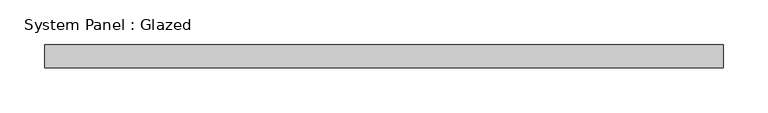
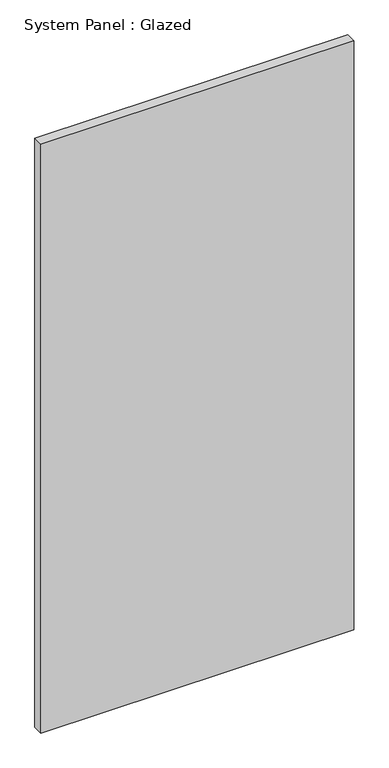
"""IFC4 building model written with IfcOpenShell, lengths in millimetres: plate geometry, System Panel : Glazed."""

from ifc_helpers import new_model, si_unit, origin, origin_with_axes, place, context, project, spatial, polyline, outline, extrude, source, transform, mapped, element, save


def system_panel_glazed_d3b8a183(model_context):
    return source(origin(), model_context, "Body", "SweptSolid", [
        extrude(outline(polyline([(377.825, 19.05), (-377.825, 19.05), (-377.825, 44.45), (377.825, 44.45), (377.825, 19.05)])), origin_with_axes(), (0.0, 0.0, 1.0), 1503.7489674),
    ])


if __name__ == "__main__":
    model = new_model("IFC4")
    model_context = context("Model", 3, world=origin())
    ifc_project = project(units=[si_unit("LENGTHUNIT", "METRE", prefix="MILLI")], contexts=[model_context])
    site = spatial("IfcSite", under=ifc_project)
    building = spatial("IfcBuilding", under=site)
    placement = place(None, origin())
    system_panel_glazed_shape = system_panel_glazed_d3b8a183(model_context)
    element("IfcPlate", 1, ObjectType="System Panel : Glazed", at=placement, inside=building, context=model_context, shape_type="MappedRepresentation", body=[
        mapped(system_panel_glazed_shape, transform((0.0, 0.0, 0.0), x_axis=(1.0, 0.0, 0.0), y_axis=(0.0, 1.0, 0.0), z_axis=(0.0, 0.0, 1.0))),
    ])
    save(model, "model.ifc")

# Revit data of these elements
# Type "System Panel : Glazed"
#   Construction Type Id = "GSP4R"
#   Analytic Construction = "1/8 in Pilkington single glazing"
#   Visual Light Transmittance = 0.9
#   Solar Heat Gain Coefficient = 0.86
#   Heat Transfer Coefficient (U) = 1.18115 BTU/(h·ft²·°F)
#   Define Thermal Properties by = 1
# Element 1 (IfcPlate, "System Panel : Glazed")
#   Materials on its faces: "Glass"
# Materials
#   "Glass": class "Glass", colour RGB 0 128 192, transparency 0.75, Description = "Soda Lime Glass", Cost = 0
